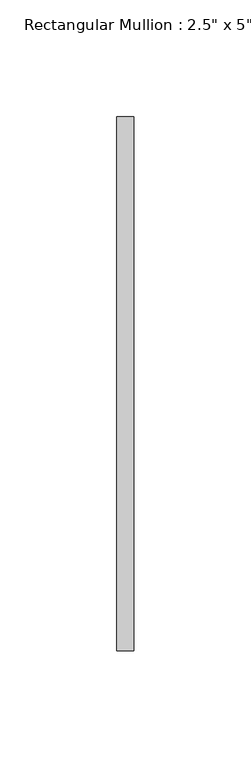
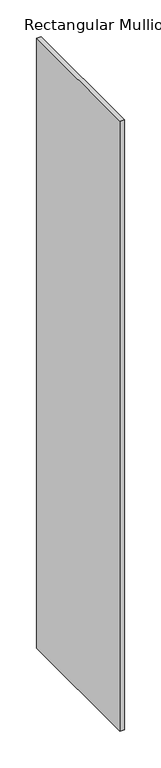
"""IFC4 building model written with IfcOpenShell, lengths in millimetres: member geometry."""

from ifc_helpers import new_model, si_unit, frame, origin, place, context, project, spatial, polyline, outline, extrude, source, transform, mapped, element, save


def member_46601aaa(model_context):
    return source(origin(), model_context, "Body", "SweptSolid", [
        extrude(outline(polyline([(0.0, 114.3), (0.0, -114.3), (-7.239, -114.3), (-7.239, 114.3), (0.0, 114.3)])), frame((0.0, 0.0, -1017.8415), z_axis=(0.0, 0.0, 1.0), x_axis=(1.0, 0.0, 0.0)), (0.0, 0.0, 1.0), 1017.8415),
    ])


if __name__ == "__main__":
    model = new_model("IFC4")
    model_context = context("Model", 3, world=origin())
    ifc_project = project(units=[si_unit("LENGTHUNIT", "METRE", prefix="MILLI")], contexts=[model_context])
    site = spatial("IfcSite", under=ifc_project)
    building = spatial("IfcBuilding", under=site)
    placement = place(None, origin())
    member_shape = member_46601aaa(model_context)
    element("IfcMember", 1, ObjectType="Rectangular Mullion : 2.5\" x 5\" rectangular", at=placement, inside=building, context=model_context, shape_type="MappedRepresentation", body=[
        mapped(member_shape, transform((0.0, 0.0, 0.0), x_axis=(1.0, 0.0, 0.0), y_axis=(0.0, 1.0, 0.0), z_axis=(0.0, 0.0, 1.0))),
    ])
    save(model, "model.ifc")

# Revit data of these elements
# Type "Rectangular Mullion : 2.5\" x 5\" rectangular"
#   built-in parameter 1007304 = 0.75 (stored number, unit not read)
#   built-in parameter 1007301 = 0.011875 (stored number, unit not read)
#   built-in parameter 1007300 = 0.011875 (stored number, unit not read)
# Element 1 (IfcMember, "Rectangular Mullion : 2.5\" x 5\" rectangular")
#   Materials on its faces: "WINDOW GLASS MATERIAL"
# Materials
#   "WINDOW GLASS MATERIAL": class "Generic", colour RGB 120 120 120, transparency 0, Cost = 0
